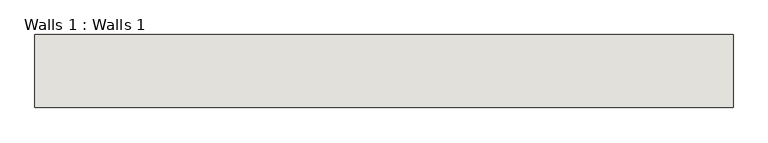
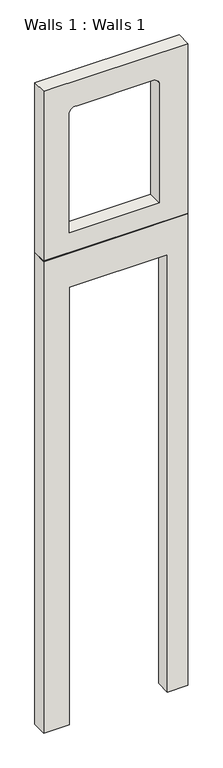
"""IFC4 building model written with IfcOpenShell, lengths in millimetres: wall geometry, Walls 1 : Walls 1."""

from ifc_helpers import new_model, si_unit, point, frame, frame_2d, origin, place, context, project, spatial, polyline, circle_curve, trimmed, segment, composite_curve, outline, extrude, source, transform, mapped, element, save


def walls_1_walls_1_151b54a8(model_context):
    return source(origin(), model_context, "Body", "SweptSolid", [
        extrude(outline(polyline([(14935.2, -5851.4998814), (14935.2, -9026.4998814), (10985.8175121, -9026.4998814), (10985.8175121, -5851.4998814), (14935.2, -5851.4998814)]), holes=[composite_curve([segment(trimmed(circle_curve(frame_2d((14207.1312748, -8325.2227377)), 134.540625), [point((14207.1312748, -8459.7633627))], [point((14340.4812748, -8307.3633627))], True, "CARTESIAN"), True, "CONTINUOUS"), segment(polyline([(14340.4812748, -8307.3633627), (14340.4812748, -6630.9633627)]), True, "CONTINUOUS"), segment(trimmed(circle_curve(frame_2d((14176.5725766, -6630.9633627)), 163.9086982), [point((14340.4812748, -6630.9633627))], [point((14236.9074865, -6478.5633627))], True, "CARTESIAN"), True, "CONTINUOUS"), segment(polyline([(14236.9074865, -6478.5633627), (11444.8812748, -6478.5633627), (11444.8812748, -8459.7633627), (14207.1312748, -8459.7633627)]), True, "CONTINUOUS")], self_intersect=False)]), frame((0.0, -57.4389176, 0.0), z_axis=(0.0, 1.0, 0.0), x_axis=(0.0, 0.0, 1.0)), (0.0, 0.0, 1.0), 330.2),
        extrude(outline(polyline([(10972.8, -5851.4998814), (10972.8, -9026.4998814), (0.0, -9026.4998814), (0.0, -8459.7633627), (10181.7801403, -8459.7633627), (10181.7801403, -6301.343851), (0.0, -6301.343851), (0.0, -5851.4998814), (10972.8, -5851.4998814)])), frame((0.0, -57.4389176, 0.0), z_axis=(0.0, 1.0, 0.0), x_axis=(0.0, 0.0, 1.0)), (0.0, 0.0, 1.0), 330.2),
    ])


if __name__ == "__main__":
    model = new_model("IFC4")
    model_context = context("Model", 3, world=origin())
    ifc_project = project(units=[si_unit("LENGTHUNIT", "METRE", prefix="MILLI")], contexts=[model_context])
    site = spatial("IfcSite", under=ifc_project)
    building = spatial("IfcBuilding", under=site)
    placement = place(None, origin())
    walls_1_walls_1_shape = walls_1_walls_1_151b54a8(model_context)
    element("IfcWall", 1, ObjectType="Walls 1 : Walls 1", at=placement, inside=building, context=model_context, shape_type="MappedRepresentation", body=[
        mapped(walls_1_walls_1_shape, transform((0.0, 0.0, 0.0), x_axis=(1.0, 0.0, 0.0), y_axis=(0.0, 1.0, 0.0), z_axis=(0.0, 0.0, 1.0))),
    ])
    save(model, "model.ifc")

# Revit data of these elements
# Element 1 (IfcWall, "Walls 1 : Walls 1")
#   Materials on its faces: "Default Wall"
# Materials
#   "Default Wall": colour RGB 128 128 128, transparency 0
